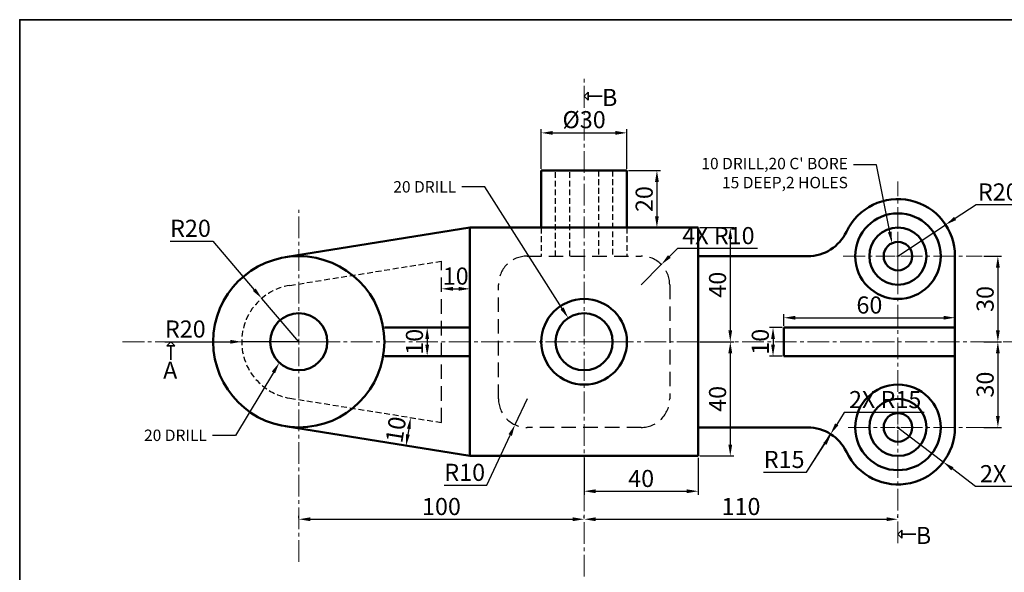
# Model space of a CAD drawing. Units: millimetres. Extents: x 33 to 569, y -180 to 232.
# Tile 2 of 3: x 33 to 378, y 39 to 232. Entities that reach past the tile are written whole.
import ezdxf
from ezdxf import colors
from ezdxf.entities.mleader import LeaderData, LeaderLine
from ezdxf.math import Vec2, Vec3

# ---------------------------------------------------------------- set-up
doc = ezdxf.new("R2010")
doc.units = ezdxf.units.MM
doc.header["$LTSCALE"] = 0.4
doc.linetypes.add('CENTER2', pattern=[28.575, 19.05, -3.175, 3.175, -3.175])
doc.linetypes.add('DASHED', pattern=[19.05, 12.7, -6.35])
for name, color, linetype, lineweight in [('M-CNTR', 1, 'CENTER2', 18), ('M-DIMS', 2, 'Continuous', 25), ('M-HIDN', 4, 'DASHED', 25), ('M-OUTL', 7, 'Continuous', 50), ('M-SECT', 6, 'Continuous', 35), ('M-TEXT', 3, 'Continuous', 25), ('M-TTLB', 7, 'Continuous', 35)]:
    doc.layers.add(name, color=color, linetype=linetype, lineweight=lineweight)
doc.styles.get("Standard").update_dxf_attribs({"font": 'arial.ttf'})
doc.dimstyles.new('ISO-25', dxfattribs={"dimtxt": 6, "dimasz": 4, "dimexe": 1.25, "dimexo": 0.625, "dimtad": 1, "dimtoh": 1, "dimdec": 0, "dimtxsty": 'Standard', "dimcen": 2.5, "dimadec": 0, "dimazin": 0, "dimtfac": 1, "dimtdec": 0, "dimtmove": 0, "dimatfit": 3, "dimfxl": 1, "dimarcsym": 0})

# ---------------------------------------------------------------- blocks, each defined once
blk = doc.blocks.new('*U1')
at = {"layer": 'M-CNTR', "color": 0, "transparency": 16777216}
blk.add_line((-161.75, 0), (175, 0), dxfattribs=at)
blk = doc.blocks.new('*U2')
at = {"layer": 'M-CNTR', "color": 0, "transparency": 16777216}
for p, q in [((0, 2), (0, 92.17)), ((-13.5, 0), (-2, 0)), ((2, 0), (13.5, 0)), ((0, -219.39), (0, -2))]:
    blk.add_line(p, q, dxfattribs=at)
at = {"layer": 'M-CNTR', "color": 0, "linetype": 'Continuous', "transparency": 16777216}
for p, q in [((-1, 0), (1, 0)), ((0, -1), (0, 1))]:
    blk.add_line(p, q, dxfattribs=at)
blk = doc.blocks.new('*U3')
at = {"layer": 'M-CNTR', "color": 0, "transparency": 16777216}
for p, q in [((0, 1), (0, 86.19)), ((-17.49, 0), (-1, 0)), ((1, 0), (30.13, 0)), ((0, -40.58), (0, -1))]:
    blk.add_line(p, q, dxfattribs=at)
at = {"layer": 'M-CNTR', "color": 0, "linetype": 'Continuous', "transparency": 16777216}
for p, q in [((-0.5, 0), (0.5, 0)), ((0, -0.5), (0, 0.5))]:
    blk.add_line(p, q, dxfattribs=at)
blk = doc.blocks.new('*D4')
at = {"layer": 'Defpoints', "color": 0, "ltscale": 0.4, "transparency": 16777216}
for p in [(245.35, 179.63), (245.35, 159.63), (255.87, 159.63)]:
    blk.add_point(p, dxfattribs=at)
at = {"layer": 'M-DIMS', "color": 0, "lineweight": -2, "ltscale": 0.4, "transparency": 16777216}
for p, q in [((245.97, 179.63), (257.12, 179.63)), ((255.87, 175.63), (255.87, 163.63)), ((245.97, 159.63), (257.12, 159.63))]:
    blk.add_line(p, q, dxfattribs=at)
at = {"layer": 'M-DIMS', "color": 0, "ltscale": 0.4, "transparency": 16777216}
for points in [[(255.2, 175.63), (256.54, 175.63), (255.87, 179.63)], [(255.2, 163.63), (256.54, 163.63), (255.87, 159.63)]]:
    blk.add_solid(points, dxfattribs=at)
at = {"layer": 'M-DIMS', "color": 0, "ltscale": 0.4, "transparency": 16777216, "insert": (252.18, 169.63), "char_height": 6, "attachment_point": 5, "rotation": 90}
blk.add_mtext('20', dxfattribs=at)
blk = doc.blocks.new('*D5')
at = {"layer": 'Defpoints', "color": 0, "ltscale": 0.4, "transparency": 16777216}
for p in [(245.35, 192.83), (215.35, 179.63), (245.35, 179.63)]:
    blk.add_point(p, dxfattribs=at)
at = {"layer": 'M-DIMS', "color": 0, "lineweight": -2, "ltscale": 0.4, "transparency": 16777216}
for p, q in [((215.35, 180.25), (215.35, 194.08)), ((245.35, 180.25), (245.35, 194.08)), ((219.35, 192.83), (241.35, 192.83))]:
    blk.add_line(p, q, dxfattribs=at)
at = {"layer": 'M-DIMS', "color": 0, "ltscale": 0.4, "transparency": 16777216}
for points in [[(219.35, 193.49), (219.35, 192.16), (215.35, 192.83)], [(241.35, 193.49), (241.35, 192.16), (245.35, 192.83)]]:
    blk.add_solid(points, dxfattribs=at)
at = {"layer": 'M-DIMS', "color": 0, "ltscale": 0.4, "transparency": 16777216, "insert": (230.35, 196.68), "char_height": 6, "attachment_point": 5}
blk.add_mtext('%%C30', dxfattribs=at)
blk = doc.blocks.new('*D6')
at = {"layer": 'Defpoints', "color": 0, "ltscale": 0.4, "transparency": 16777216}
for p in [(180.35, 138.19), (190.35, 138.19), (190.35, 138.19)]:
    blk.add_point(p, dxfattribs=at)
at = {"layer": 'M-DIMS', "color": 0, "lineweight": -2, "ltscale": 0.4, "transparency": 16777216}
for p, q in [((180.35, 138.82), (180.35, 139.44)), ((184.35, 138.19), (186.35, 138.19)), ((190.35, 138.82), (190.35, 139.44))]:
    blk.add_line(p, q, dxfattribs=at)
at = {"layer": 'M-DIMS', "color": 0, "ltscale": 0.4, "transparency": 16777216}
for points in [[(184.35, 138.86), (184.35, 137.52), (180.35, 138.19)], [(186.35, 138.86), (186.35, 137.52), (190.35, 138.19)]]:
    blk.add_solid(points, dxfattribs=at)
at = {"layer": 'M-DIMS', "color": 0, "ltscale": 0.4, "transparency": 16777216, "insert": (185.35, 141.88), "char_height": 6, "attachment_point": 5}
blk.add_mtext('10', dxfattribs=at)
blk = doc.blocks.new('*D7')
at = {"layer": 'Defpoints', "color": 0, "ltscale": 0.4, "transparency": 16777216}
for p in [(175.35, 124.63), (175.35, 114.63), (175.35, 114.63)]:
    blk.add_point(p, dxfattribs=at)
at = {"layer": 'M-DIMS', "color": 0, "lineweight": -2, "ltscale": 0.4, "transparency": 16777216}
for p, q in [((175.97, 124.63), (176.6, 124.63)), ((175.35, 120.63), (175.35, 118.63)), ((175.97, 114.63), (176.6, 114.63))]:
    blk.add_line(p, q, dxfattribs=at)
at = {"layer": 'M-DIMS', "color": 0, "ltscale": 0.4, "transparency": 16777216}
for points in [[(174.68, 120.63), (176.02, 120.63), (175.35, 124.63)], [(174.68, 118.63), (176.02, 118.63), (175.35, 114.63)]]:
    blk.add_solid(points, dxfattribs=at)
at = {"layer": 'M-DIMS', "color": 0, "ltscale": 0.4, "transparency": 16777216, "insert": (171.66, 119.63), "char_height": 6, "attachment_point": 5, "rotation": 90}
blk.add_mtext('10', dxfattribs=at)
blk = doc.blocks.new('*D8')
at = {"layer": 'Defpoints', "color": 0, "ltscale": 0.4, "transparency": 16777216}
for p in [(270.35, 159.63), (270.35, 119.63), (281.59, 119.63)]:
    blk.add_point(p, dxfattribs=at)
at = {"layer": 'M-DIMS', "color": 0, "lineweight": -2, "ltscale": 0.4, "transparency": 16777216}
for p, q in [((270.97, 159.63), (282.84, 159.63)), ((281.59, 155.63), (281.59, 123.63)), ((270.97, 119.63), (282.84, 119.63))]:
    blk.add_line(p, q, dxfattribs=at)
at = {"layer": 'M-DIMS', "color": 0, "ltscale": 0.4, "transparency": 16777216}
for points in [[(280.92, 155.63), (282.25, 155.63), (281.59, 159.63)], [(280.92, 123.63), (282.25, 123.63), (281.59, 119.63)]]:
    blk.add_solid(points, dxfattribs=at)
at = {"layer": 'M-DIMS', "color": 0, "ltscale": 0.4, "transparency": 16777216, "insert": (277.9, 139.63), "char_height": 6, "attachment_point": 5, "rotation": 90}
blk.add_mtext('40', dxfattribs=at)
blk = doc.blocks.new('*D9')
at = {"layer": 'Defpoints', "color": 0, "ltscale": 0.4, "transparency": 16777216}
for p in [(270.35, 119.63), (270.35, 79.63), (281.59, 79.63)]:
    blk.add_point(p, dxfattribs=at)
at = {"layer": 'M-DIMS', "color": 0, "lineweight": -2, "ltscale": 0.4, "transparency": 16777216}
for p, q in [((270.97, 119.63), (282.84, 119.63)), ((281.59, 115.63), (281.59, 83.63)), ((270.97, 79.63), (282.84, 79.63))]:
    blk.add_line(p, q, dxfattribs=at)
at = {"layer": 'M-DIMS', "color": 0, "ltscale": 0.4, "transparency": 16777216}
for points in [[(280.92, 115.63), (282.25, 115.63), (281.59, 119.63)], [(280.92, 83.63), (282.25, 83.63), (281.59, 79.63)]]:
    blk.add_solid(points, dxfattribs=at)
at = {"layer": 'M-DIMS', "color": 0, "ltscale": 0.4, "transparency": 16777216, "insert": (277.9, 99.63), "char_height": 6, "attachment_point": 5, "rotation": 90}
blk.add_mtext('40', dxfattribs=at)
blk = doc.blocks.new('*D10')
at = {"layer": 'Defpoints', "color": 0, "ltscale": 0.4, "transparency": 16777216}
for p in [(300.35, 124.63), (296.57, 114.63), (300.35, 114.63)]:
    blk.add_point(p, dxfattribs=at)
at = {"layer": 'M-DIMS', "color": 0, "lineweight": -2, "ltscale": 0.4, "transparency": 16777216}
for p, q in [((299.72, 124.63), (295.32, 124.63)), ((296.57, 120.63), (296.57, 118.63)), ((299.72, 114.63), (295.32, 114.63))]:
    blk.add_line(p, q, dxfattribs=at)
at = {"layer": 'M-DIMS', "color": 0, "ltscale": 0.4, "transparency": 16777216}
for points in [[(295.9, 120.63), (297.24, 120.63), (296.57, 124.63)], [(295.9, 118.63), (297.24, 118.63), (296.57, 114.63)]]:
    blk.add_solid(points, dxfattribs=at)
at = {"layer": 'M-DIMS', "color": 0, "ltscale": 0.4, "transparency": 16777216, "insert": (292.88, 119.63), "char_height": 6, "attachment_point": 5, "rotation": 90}
blk.add_mtext('10', dxfattribs=at)
blk = doc.blocks.new('*D11')
at = {"layer": 'Defpoints', "color": 0, "ltscale": 0.4, "transparency": 16777216}
for p in [(360.35, 128.05), (300.35, 124.63), (360.35, 124.63)]:
    blk.add_point(p, dxfattribs=at)
at = {"layer": 'M-DIMS', "color": 0, "lineweight": -2, "ltscale": 0.4, "transparency": 16777216}
for p, q in [((300.35, 125.25), (300.35, 129.3)), ((304.35, 128.05), (356.35, 128.05)), ((360.35, 125.25), (360.35, 129.3))]:
    blk.add_line(p, q, dxfattribs=at)
at = {"layer": 'M-DIMS', "color": 0, "ltscale": 0.4, "transparency": 16777216}
for points in [[(304.35, 128.72), (304.35, 127.39), (300.35, 128.05)], [(356.35, 128.72), (356.35, 127.39), (360.35, 128.05)]]:
    blk.add_solid(points, dxfattribs=at)
at = {"layer": 'M-DIMS', "color": 0, "ltscale": 0.4, "transparency": 16777216, "insert": (330.35, 131.74), "char_height": 6, "attachment_point": 5}
blk.add_mtext('60', dxfattribs=at)
blk = doc.blocks.new('*D12')
at = {"layer": 'Defpoints', "color": 0, "ltscale": 0.4, "transparency": 16777216}
for p in [(230.35, 79.63), (270.35, 79.63), (270.35, 67.27)]:
    blk.add_point(p, dxfattribs=at)
at = {"layer": 'M-DIMS', "color": 0, "lineweight": -2, "ltscale": 0.4, "transparency": 16777216}
for p, q in [((230.35, 79), (230.35, 66.02)), ((270.35, 79), (270.35, 66.02)), ((234.35, 67.27), (266.35, 67.27))]:
    blk.add_line(p, q, dxfattribs=at)
at = {"layer": 'M-DIMS', "color": 0, "ltscale": 0.4, "transparency": 16777216}
for points in [[(234.35, 67.93), (234.35, 66.6), (230.35, 67.27)], [(266.35, 67.93), (266.35, 66.6), (270.35, 67.27)]]:
    blk.add_solid(points, dxfattribs=at)
at = {"layer": 'M-DIMS', "color": 0, "ltscale": 0.4, "transparency": 16777216, "insert": (250.35, 70.95), "char_height": 6, "attachment_point": 5}
blk.add_mtext('40', dxfattribs=at)
blk = doc.blocks.new('*U13')
at = {"layer": 'M-CNTR', "color": 0, "transparency": 16777216}
for p, q in [((0, 2), (0, 46.22)), ((-13.5, 0), (-2, 0)), ((2, 0), (13.5, 0)), ((0, -77.08), (0, -2))]:
    blk.add_line(p, q, dxfattribs=at)
at = {"layer": 'M-CNTR', "color": 0, "linetype": 'Continuous', "transparency": 16777216}
for p, q in [((-1, 0), (1, 0)), ((0, -1), (0, 1))]:
    blk.add_line(p, q, dxfattribs=at)
blk = doc.blocks.new('*D14')
at = {"layer": 'Defpoints', "color": 0, "ltscale": 0.4, "transparency": 16777216}
for p in [(130.35, 57.22), (230.35, 57.45), (230.35, 57.22)]:
    blk.add_point(p, dxfattribs=at)
at = {"layer": 'M-DIMS', "color": 0, "lineweight": -2, "ltscale": 0.4, "transparency": 16777216}
for p, q in [((130.35, 57.85), (130.35, 58.7)), ((230.35, 57.85), (230.35, 58.7)), ((134.35, 57.45), (226.35, 57.45))]:
    blk.add_line(p, q, dxfattribs=at)
at = {"layer": 'M-DIMS', "color": 0, "ltscale": 0.4, "transparency": 16777216}
for points in [[(134.35, 58.12), (134.35, 56.78), (130.35, 57.45)], [(226.35, 58.12), (226.35, 56.78), (230.35, 57.45)]]:
    blk.add_solid(points, dxfattribs=at)
at = {"layer": 'M-DIMS', "color": 0, "ltscale": 0.4, "transparency": 16777216, "insert": (180.35, 61.14), "char_height": 6, "attachment_point": 5}
blk.add_mtext('100', dxfattribs=at)
blk = doc.blocks.new('*D15')
at = {"layer": 'Defpoints', "color": 0, "ltscale": 0.4, "transparency": 16777216}
for p in [(230.35, 57.45), (340.35, 57.45), (340.35, 57.45)]:
    blk.add_point(p, dxfattribs=at)
at = {"layer": 'M-DIMS', "color": 0, "lineweight": -2, "ltscale": 0.4, "transparency": 16777216}
for p, q in [((230.35, 58.08), (230.35, 58.7)), ((340.35, 58.08), (340.35, 58.7)), ((234.35, 57.45), (336.35, 57.45))]:
    blk.add_line(p, q, dxfattribs=at)
at = {"layer": 'M-DIMS', "color": 0, "ltscale": 0.4, "transparency": 16777216}
for points in [[(234.35, 58.12), (234.35, 56.78), (230.35, 57.45)], [(336.35, 58.12), (336.35, 56.78), (340.35, 57.45)]]:
    blk.add_solid(points, dxfattribs=at)
at = {"layer": 'M-DIMS', "color": 0, "ltscale": 0.4, "transparency": 16777216, "insert": (285.35, 61.14), "char_height": 6, "attachment_point": 5}
blk.add_mtext('110', dxfattribs=at)
blk = doc.blocks.new('*U16')
at = {"layer": 'M-CNTR', "color": 0, "transparency": 16777216}
for p, q in [((0, 1), (0, 8.5)), ((-19.15, 0), (-1, 0)), ((1, 0), (29.5, 0)), ((0, -8.5), (0, -1))]:
    blk.add_line(p, q, dxfattribs=at)
at = {"layer": 'M-CNTR', "color": 0, "linetype": 'Continuous', "transparency": 16777216}
for p, q in [((-0.5, 0), (0.5, 0)), ((0, -0.5), (0, 0.5))]:
    blk.add_line(p, q, dxfattribs=at)
blk = doc.blocks.new('*D17')
at = {"layer": 'Defpoints', "color": 0, "ltscale": 0.4, "transparency": 16777216}
for p in [(369.85, 149.63), (369.85, 119.63), (375.38, 119.63)]:
    blk.add_point(p, dxfattribs=at)
at = {"layer": 'M-DIMS', "color": 0, "lineweight": -2, "ltscale": 0.4, "transparency": 16777216}
for p, q in [((370.47, 149.63), (376.63, 149.63)), ((375.38, 145.63), (375.38, 123.63)), ((370.47, 119.63), (376.63, 119.63))]:
    blk.add_line(p, q, dxfattribs=at)
at = {"layer": 'M-DIMS', "color": 0, "ltscale": 0.4, "transparency": 16777216}
for points in [[(374.71, 145.63), (376.04, 145.63), (375.38, 149.63)], [(374.71, 123.63), (376.04, 123.63), (375.38, 119.63)]]:
    blk.add_solid(points, dxfattribs=at)
at = {"layer": 'M-DIMS', "color": 0, "ltscale": 0.4, "transparency": 16777216, "insert": (371.69, 134.63), "char_height": 6, "attachment_point": 5, "rotation": 90}
blk.add_mtext('30', dxfattribs=at)
blk = doc.blocks.new('*D18')
at = {"layer": 'Defpoints', "color": 0, "ltscale": 0.4, "transparency": 16777216}
for p in [(369.85, 119.63), (369.85, 89.63), (375.38, 89.63)]:
    blk.add_point(p, dxfattribs=at)
at = {"layer": 'M-DIMS', "color": 0, "lineweight": -2, "ltscale": 0.4, "transparency": 16777216}
for p, q in [((370.47, 119.63), (376.63, 119.63)), ((375.38, 115.63), (375.38, 93.63)), ((370.47, 89.63), (376.63, 89.63))]:
    blk.add_line(p, q, dxfattribs=at)
at = {"layer": 'M-DIMS', "color": 0, "ltscale": 0.4, "transparency": 16777216}
for points in [[(374.71, 115.63), (376.04, 115.63), (375.38, 119.63)], [(374.71, 93.63), (376.04, 93.63), (375.38, 89.63)]]:
    blk.add_solid(points, dxfattribs=at)
at = {"layer": 'M-DIMS', "color": 0, "ltscale": 0.4, "transparency": 16777216, "insert": (371.69, 104.63), "char_height": 6, "attachment_point": 5, "rotation": 90}
blk.add_mtext('30', dxfattribs=at)
blk = doc.blocks.new('*D19')
at = {"layer": 'Defpoints', "color": 0, "ltscale": 0.4, "transparency": 16777216}
for p in [(357.05, 160.63), (340.35, 149.63)]:
    blk.add_point(p, dxfattribs=at)
at = {"layer": 'M-DIMS', "color": 0, "lineweight": -2, "ltscale": 0.4, "transparency": 16777216}
for p, q in [((367.74, 167.66), (360.4, 162.83)), ((382.68, 167.66), (367.74, 167.66)), ((340.35, 149.63), (357.05, 160.63))]:
    blk.add_line(p, q, dxfattribs=at)
at = {"layer": 'M-DIMS', "color": 0, "ltscale": 0.4, "transparency": 16777216}
blk.add_solid([(360.03, 163.38), (360.76, 162.27), (357.05, 160.63)], dxfattribs=at)
at = {"layer": 'M-DIMS', "color": 0, "ltscale": 0.4, "transparency": 16777216, "insert": (375.52, 171.35), "char_height": 6, "attachment_point": 5}
blk.add_mtext('R20', dxfattribs=at)
blk = doc.blocks.new('*D20')
at = {"layer": 'Defpoints', "color": 0, "ltscale": 0.4, "transparency": 16777216}
for p in [(210.35, 99.63), (206.13, 90.56)]:
    blk.add_point(p, dxfattribs=at)
at = {"layer": 'M-DIMS', "color": 0, "lineweight": -2, "ltscale": 0.4, "transparency": 16777216}
for p, q in [((210.35, 99.63), (206.13, 90.56)), ((196.28, 69.42), (204.44, 86.94)), ((181.34, 69.42), (196.28, 69.42))]:
    blk.add_line(p, q, dxfattribs=at)
at = {"layer": 'M-DIMS', "color": 0, "ltscale": 0.4, "transparency": 16777216}
blk.add_solid([(203.84, 87.22), (205.04, 86.66), (206.13, 90.56)], dxfattribs=at)
at = {"layer": 'M-DIMS', "color": 0, "ltscale": 0.4, "transparency": 16777216, "insert": (188.5, 73.11), "char_height": 6, "attachment_point": 5}
blk.add_mtext('R10', dxfattribs=at)
blk = doc.blocks.new('*D21')
at = {"layer": 'Defpoints', "color": 0, "ltscale": 0.4, "transparency": 16777216}
for p in [(316.92, 87.19), (308.73, 74.63)]:
    blk.add_point(p, dxfattribs=at)
at = {"layer": 'M-DIMS', "color": 0, "lineweight": -2, "ltscale": 0.4, "transparency": 16777216}
for p, q in [((308.28, 73.95), (314.74, 83.84)), ((293.27, 73.95), (308.28, 73.95))]:
    blk.add_line(p, q, dxfattribs=at)
at = {"layer": 'M-DIMS', "color": 0, "ltscale": 0.4, "transparency": 16777216}
blk.add_solid([(314.18, 84.21), (315.29, 83.48), (316.92, 87.19)], dxfattribs=at)
at = {"layer": 'M-DIMS', "color": 0, "ltscale": 0.4, "transparency": 16777216, "insert": (300.47, 77.63), "char_height": 6, "attachment_point": 5}
blk.add_mtext('R15', dxfattribs=at)
blk = doc.blocks.new('*D22')
at = {"layer": 'Defpoints', "color": 0, "ltscale": 0.4, "transparency": 16777216}
for p in [(117.36, 134.83), (130.35, 119.63)]:
    blk.add_point(p, dxfattribs=at)
at = {"layer": 'M-DIMS', "color": 0, "lineweight": -2, "ltscale": 0.4, "transparency": 16777216}
for p, q in [((85.24, 154.93), (100.18, 154.93)), ((100.18, 154.93), (114.76, 137.87)), ((130.35, 119.63), (117.36, 134.83))]:
    blk.add_line(p, q, dxfattribs=at)
at = {"layer": 'M-DIMS', "color": 0, "ltscale": 0.4, "transparency": 16777216}
blk.add_solid([(115.26, 138.31), (114.25, 137.44), (117.36, 134.83)], dxfattribs=at)
at = {"layer": 'M-DIMS', "color": 0, "ltscale": 0.4, "transparency": 16777216, "insert": (92.39, 158.62), "char_height": 6, "attachment_point": 5}
blk.add_mtext('R20', dxfattribs=at)
blk = doc.blocks.new('*D23')
at = {"layer": 'Defpoints', "color": 0, "ltscale": 0.4, "transparency": 16777216}
for p in [(169.55, 93.09), (167.97, 83.22), (167.97, 83.22)]:
    blk.add_point(p, dxfattribs=at)
at = {"layer": 'M-DIMS', "color": 0, "lineweight": -2, "ltscale": 0.4, "transparency": 16777216}
for p, q in [((170.17, 92.99), (170.79, 92.89)), ((168.92, 89.14), (168.6, 87.17)), ((168.59, 83.12), (169.2, 83.02))]:
    blk.add_line(p, q, dxfattribs=at)
at = {"layer": 'M-DIMS', "color": 0, "ltscale": 0.4, "transparency": 16777216}
for points in [[(168.26, 89.25), (169.58, 89.04), (169.55, 93.09)], [(167.94, 87.27), (169.26, 87.06), (167.97, 83.22)]]:
    blk.add_solid(points, dxfattribs=at)
at = {"layer": 'M-DIMS', "color": 0, "ltscale": 0.4, "transparency": 16777216, "insert": (165.12, 88.74), "char_height": 6, "attachment_point": 5, "rotation": 80.8938}
blk.add_mtext('10', dxfattribs=at)
blk = doc.blocks.new('SECTION-ARROW')
at = {"ltscale": 0.4}
for p, q in [((0, 1.41), (1.41, 2.83)), ((0, 1.41), (1.41, 0)), ((1.41, 2.83), (1.41, 0)), ((1.41, 1.41), (6.28, 1.41))]:
    blk.add_line(p, q, dxfattribs=at)
blk = doc.blocks.new('CBORE-M10')
for radius in [15, 10, 5]:
    blk.add_circle((15, 15), radius)
blk = doc.blocks.new('*D49')
at = {"layer": 'Defpoints', "color": 0, "ltscale": 0.4, "transparency": 16777216}
for p in [(340.35, 89.63), (356.26, 77.51)]:
    blk.add_point(p, dxfattribs=at)
at = {"layer": 'M-DIMS', "color": 0, "lineweight": -2, "ltscale": 0.4, "transparency": 16777216}
for p, q in [((340.35, 89.63), (356.26, 77.51)), ((367.5, 68.95), (359.44, 75.09)), ((395.43, 68.95), (367.5, 68.95))]:
    blk.add_line(p, q, dxfattribs=at)
at = {"layer": 'M-DIMS', "color": 0, "ltscale": 0.4, "transparency": 16777216}
blk.add_solid([(359.85, 75.62), (359.04, 74.56), (356.26, 77.51)], dxfattribs=at)
at = {"layer": 'M-DIMS', "color": 0, "ltscale": 0.4, "transparency": 16777216, "insert": (381.78, 72.64), "char_height": 6, "attachment_point": 5}
blk.add_mtext('2X R20', dxfattribs=at)
blk = doc.blocks.new('*D50')
at = {"layer": 'Defpoints', "color": 0, "ltscale": 0.4, "transparency": 16777216}
for p in [(316.74, 87.31), (308.73, 74.63)]:
    blk.add_point(p, dxfattribs=at)
at = {"layer": 'M-DIMS', "color": 0, "lineweight": -2, "ltscale": 0.4, "transparency": 16777216}
for p, q in [((321.56, 94.91), (318.88, 90.69)), ((349.56, 94.91), (321.56, 94.91)), ((308.73, 74.63), (316.74, 87.31))]:
    blk.add_line(p, q, dxfattribs=at)
at = {"layer": 'M-DIMS', "color": 0, "ltscale": 0.4, "transparency": 16777216}
blk.add_solid([(318.32, 91.04), (319.45, 90.33), (316.74, 87.31)], dxfattribs=at)
at = {"layer": 'M-DIMS', "color": 0, "ltscale": 0.4, "transparency": 16777216, "insert": (335.87, 98.6), "char_height": 6, "attachment_point": 5}
blk.add_mtext('2X R15', dxfattribs=at)
blk = doc.blocks.new('*D51')
at = {"layer": 'Defpoints', "color": 0, "ltscale": 0.4, "transparency": 16777216}
for p in [(257.42, 146.7), (250.35, 139.63)]:
    blk.add_point(p, dxfattribs=at)
at = {"layer": 'M-DIMS', "color": 0, "lineweight": -2, "ltscale": 0.4, "transparency": 16777216}
for p, q in [((263.08, 152.36), (260.25, 149.53)), ((291.15, 152.36), (263.08, 152.36)), ((250.35, 139.63), (257.42, 146.7))]:
    blk.add_line(p, q, dxfattribs=at)
at = {"layer": 'M-DIMS', "color": 0, "ltscale": 0.4, "transparency": 16777216}
blk.add_solid([(259.78, 150), (260.72, 149.06), (257.42, 146.7)], dxfattribs=at)
at = {"layer": 'M-DIMS', "color": 0, "ltscale": 0.4, "transparency": 16777216, "insert": (277.43, 156.05), "char_height": 6, "attachment_point": 5}
blk.add_mtext('4X R10', dxfattribs=at)
blk = doc.blocks.new('*D52')
at = {"layer": 'Defpoints', "color": 0, "ltscale": 0.4, "transparency": 16777216}
for p in [(110.35, 119.63), (130.35, 119.63)]:
    blk.add_point(p, dxfattribs=at)
at = {"layer": 'M-DIMS', "color": 0, "lineweight": -2, "ltscale": 0.4, "transparency": 16777216}
for p, q in [((83.41, 119.63), (98.35, 119.63)), ((98.35, 119.63), (106.35, 119.63)), ((130.35, 119.63), (110.35, 119.63))]:
    blk.add_line(p, q, dxfattribs=at)
at = {"layer": 'M-DIMS', "color": 0, "ltscale": 0.4, "transparency": 16777216}
blk.add_solid([(106.35, 120.3), (106.35, 118.96), (110.35, 119.63)], dxfattribs=at)
at = {"layer": 'M-DIMS', "color": 0, "ltscale": 0.4, "transparency": 16777216, "insert": (90.57, 123.32), "char_height": 6, "attachment_point": 5}
blk.add_mtext('R20', dxfattribs=at)

msp = doc.modelspace()

# ---------------------------------------------------------------- linework, layer by layer
at = {"layer": 'M-HIDN', "ltscale": 0.4}
for p, q in [((220.35, 149.63), (220.35, 179.63)), ((225.35, 149.63), (225.35, 179.63)), ((235.35, 179.63), (235.35, 149.63)), ((240.35, 179.63), (240.35, 149.63)), ((215.35, 159.63), (215.35, 149.63)), ((245.35, 159.63), (245.35, 149.63)), ((127.18, 139.38), (180.35, 147.9)), ((127.18, 99.88), (180.35, 91.36))]:
    msp.add_line(p, q, dxfattribs=at)
at = {"layer": 'M-HIDN'}
msp.add_line((180.35, 91.36), (180.35, 147.9), dxfattribs=at)
msp.add_lwpolyline([(210.35, 149.63), (250.35, 149.63, -0.414214), (260.35, 139.63), (260.35, 99.63, -0.414214), (250.35, 89.63), (210.35, 89.63, -0.414214), (200.35, 99.63), (200.35, 139.63, -0.414214)], format="xyb", close=True, dxfattribs=at)
at = {"layer": 'M-HIDN', "ltscale": 0.4}
msp.add_arc((130.35, 119.63), 20, 99.1062, 260.8938, dxfattribs=at)
at = {"layer": 'M-OUTL', "ltscale": 0.4}
for p, q in [((215.35, 179.63), (245.35, 179.63)), ((215.35, 159.63), (215.35, 179.63)), ((245.35, 179.63), (245.35, 159.63)), ((125.6, 149.25), (190.35, 159.63)), ((245.35, 159.63), (215.35, 159.63)), ((160.35, 124.63), (190.35, 124.63)), ((300.35, 114.63), (300.35, 124.63)), ((160.35, 114.63), (190.35, 114.63)), ((125.6, 90.01), (190.35, 79.63))]:
    msp.add_line(p, q, dxfattribs=at)
at = {"layer": 'M-OUTL'}
for p, q in [((190.35, 159.63), (270.35, 159.63)), ((190.35, 79.63), (190.35, 159.63)), ((270.35, 159.63), (270.35, 79.63)), ((308.73, 149.63), (270.35, 149.63)), ((360.35, 149.63), (360.35, 89.63)), ((300.35, 124.63), (300.35, 114.63)), ((360.35, 124.63), (300.35, 124.63)), ((360.35, 114.63), (360.35, 124.63)), ((300.35, 114.63), (360.35, 114.63)), ((308.73, 89.63), (270.35, 89.63)), ((270.35, 79.63), (190.35, 79.63))]:
    msp.add_line(p, q, dxfattribs=at)
for centre, radius in [((130.35, 119.63), 30), ((230.35, 119.63), 15), ((230.35, 119.63), 10)]:
    msp.add_circle(centre, radius, dxfattribs=at)
at = {"layer": 'M-OUTL', "ltscale": 0.4}
msp.add_circle((130.35, 119.63), 10, dxfattribs=at)
at = {"layer": 'M-OUTL'}
for centre, radius, start, end in [((340.35, 149.63), 20, 0, 154.6231), ((308.73, 164.63), 15, 270, 334.6231), ((308.73, 74.63), 15, 25.3769, 90), ((340.35, 89.63), 20, 205.3769, 0)]:
    msp.add_arc(centre, radius, start, end, dxfattribs=at)
at = {"layer": 'M-TTLB', "ltscale": 0.4}
msp.add_lwpolyline([(568.64, -179.82), (32.52, -179.82), (32.52, 232.48), (568.64, 232.48)], close=True, dxfattribs=at)

# ---------------------------------------------------------------- block references
at = {"layer": 'M-CNTR'}
for name, p in [('*U2', (230.35, 119.63)), ('*U3', (340.35, 89.63)), ('*U13', (130.35, 119.63)), ('*U16', (340.35, 149.63)), ('*U1', (230.35, 119.63))]:
    msp.add_blockref(name, p, dxfattribs=at)
at = {"layer": 'M-OUTL'}
for p in [(325.35, 134.63), (325.35, 74.63)]:
    msp.add_blockref('CBORE-M10', p, dxfattribs=at)
at = {"layer": 'M-SECT'}
for p in [(230.35, 204.26), (340.35, 50.8)]:
    msp.add_blockref('SECTION-ARROW', p, dxfattribs=at)
at = {"layer": 'M-SECT', "rotation": 270.0000000000007}
msp.add_blockref('SECTION-ARROW', (84.09, 119.63), dxfattribs=at)

# ---------------------------------------------------------------- texts
at = {"layer": 'M-TEXT', "ltscale": 0.4, "char_height": 6, "attachment_point": 1}
for s, insert in [('B', (236.63, 208.23)), ('A', (82.8, 112.65)), ('B', (346.63, 54.77))]:
    msp.add_mtext_dynamic_manual_height_columns(s, width=4.1924, gutter_width=12.5, heights=[0], dxfattribs=dict(at, insert=insert))

# ---------------------------------------------------------------- dimensions: what is measured, and where the dimension line sits
at = {"layer": 'M-DIMS', "ltscale": 0.4}
dim = msp.add_linear_dim(base=(245.35, 192.83), p1=(215.35, 179.63), p2=(245.35, 179.63), text='%%C<>', dimstyle='ISO-25', override={"dimclrd": 0, "dimclre": 0, "dimclrt": 0}, dxfattribs=at)
dim.commit()
dim.dimension.update_dxf_attribs({"geometry": '*D5', "text_midpoint": (230.35, 192.83), "dimtype": 160})
for base, p1, p2, picture, middle in [((255.87, 159.63), (245.35, 179.63), (245.35, 159.63), '*D4', (252.18, 169.63)), ((281.59, 119.63), (270.35, 159.63), (270.35, 119.63), '*D8', (277.9, 139.63)), ((375.38, 119.63), (369.85, 149.63), (369.85, 119.63), '*D17', (371.69, 134.63)), ((175.35, 114.63), (175.35, 124.63), (175.35, 114.63), '*D7', (171.66, 119.63)), ((296.57, 114.63), (300.35, 124.63), (300.35, 114.63), '*D10', (292.88, 119.63)), ((281.59, 79.63), (270.35, 119.63), (270.35, 79.63), '*D9', (277.9, 99.63)), ((375.38, 89.63), (369.85, 119.63), (369.85, 89.63), '*D18', (371.69, 104.63))]:
    dim = msp.add_linear_dim(base=base, p1=p1, p2=p2, angle=90, dimstyle='ISO-25', override={"dimclrd": 0, "dimclre": 0, "dimclrt": 0}, dxfattribs=at)
    dim.commit()
    dim.dimension.update_dxf_attribs({"geometry": picture, "text_midpoint": middle})
for center, mpoint, override, picture, middle in [((340.35, 149.63), (357.05, 160.63), {"dimclrd": 0, "dimclre": 0, "dimclrt": 0}, '*D19', (375.52, 167.66)), ((130.35, 119.63), (117.36, 134.83), {"dimclrd": 0, "dimclre": 0, "dimclrt": 0}, '*D22', (92.39, 154.93)), ((130.35, 119.63), (110.35, 119.63), {"dimdec": 0, "dimlfac": 1, "dimrnd": 0, "dimzin": 0, "dimdsep": 46, "dimlunit": 2}, '*D52', (98.35, 119.63)), ((210.35, 99.63), (206.13, 90.56), {"dimclrd": 0, "dimclre": 0, "dimclrt": 0}, '*D20', (188.5, 69.42)), ((308.73, 74.63), (316.92, 87.19), {"dimclrd": 0, "dimclre": 0, "dimclrt": 0}, '*D21', (300.47, 73.95))]:
    dim = msp.add_radius_dim(center=center, mpoint=mpoint, dimstyle='ISO-25', override=override, dxfattribs=at)
    dim.commit()
    dim.dimension.update_dxf_attribs({"geometry": picture, "text_midpoint": middle, "dimtype": 164})
for center, mpoint, text, picture, middle in [((250.35, 139.63), (257.42, 146.7), '4X <>', '*D51', (277.43, 156.05)), ((340.35, 89.63), (356.26, 77.51), '2X <>', '*D49', (381.78, 72.64))]:
    dim = msp.add_radius_dim(center=center, mpoint=mpoint, text=text, dimstyle='ISO-25', override={"dimdec": 0, "dimlfac": 1, "dimrnd": 0, "dimzin": 0, "dimdsep": 46, "dimlunit": 2}, dxfattribs=at)
    dim.commit()
    dim.dimension.update_dxf_attribs({"geometry": picture, "text_midpoint": middle})
for base, p1, p2, picture, middle in [((190.35, 138.19), (180.35, 138.19), (190.35, 138.19), '*D6', (185.35, 141.88)), ((360.35, 128.05), (300.35, 124.63), (360.35, 124.63), '*D11', (330.35, 131.74)), ((270.35, 67.27), (230.35, 79.63), (270.35, 79.63), '*D12', (250.35, 70.95)), ((230.35, 57.45), (130.35, 57.22), (230.35, 57.22), '*D14', (180.35, 61.14)), ((340.35, 57.45), (230.35, 57.45), (340.35, 57.45), '*D15', (285.35, 61.14))]:
    dim = msp.add_linear_dim(base=base, p1=p1, p2=p2, dimstyle='ISO-25', override={"dimclrd": 0, "dimclre": 0, "dimclrt": 0}, dxfattribs=at)
    dim.commit()
    dim.dimension.update_dxf_attribs({"geometry": picture, "text_midpoint": middle})
dim = msp.add_radius_dim(center=(308.73, 74.63), mpoint=(316.74, 87.31), text='2X <>', dimstyle='ISO-25', override={"dimdec": 0, "dimlfac": 1, "dimrnd": 0, "dimzin": 0, "dimdsep": 46, "dimlunit": 2}, dxfattribs=at)
dim.commit()
dim.dimension.update_dxf_attribs({"geometry": '*D50', "text_midpoint": (335.87, 94.91), "dimtype": 164})
dim = msp.add_aligned_dim(p1=(169.55, 93.09), p2=(167.97, 83.22), distance=0, dimstyle='ISO-25', override={"dimclrd": 0, "dimclre": 0, "dimclrt": 0}, dxfattribs=at)
dim.commit()
dim.dimension.update_dxf_attribs({"geometry": '*D23', "text_midpoint": (165.12, 88.74)})

# ---------------------------------------------------------------- leaders
at = {"layer": 'M-TEXT', "ltscale": 0.4}
ml = msp.add_multileader_mtext('Standard', dxfattribs=at)
ml.set_content("10 DRILL,20 C' BORE\\P15 DEEP,2 HOLES", color=256)
ml.set_leader_properties()
ml.build(insert=Vec2(0, 0))
ctx = ml.context
ctx.base_point, ctx.plane_origin = Vec3(266.3, 181.68), Vec3(338.27, 154.18)
ctx.text_align_type = 2
notes = []
notes.append((ctx, [(0, (1, 1, 0), (332.81, 181.68), (-1, 0), 8, [(0, [(338.27, 154.18)], 0, [])])]))
ctx.mtext.insert, ctx.mtext.alignment, ctx.mtext.flow_direction = Vec3(322.81, 184.08), 3, 5
ml = msp.add_multileader_mtext('Standard', dxfattribs=at)
ml.set_content('20 DRILL', color=256)
ml.set_leader_properties()
ml.build(insert=Vec2(0, 0))
ctx = ml.context
ctx.base_point, ctx.plane_origin = Vec3(160.26, 173.89), Vec3(224.79, 127.94)
ctx.text_align_type = 2
notes.append((ctx, [(0, (1, 1, 0), (195.5, 173.89), (-1, 0), 8, [(0, [(224.79, 127.94)], 0, [])])]))
ctx.mtext.insert, ctx.mtext.alignment, ctx.mtext.flow_direction = Vec3(185.5, 175.93), 3, 5
ml = msp.add_multileader_mtext('Standard', dxfattribs=at)
ml.set_content('20 DRILL', color=256)
ml.set_leader_properties()
ml.build(insert=Vec2(0, 0))
ctx = ml.context
ctx.base_point, ctx.plane_origin = Vec3(72.88, 86.82), Vec3(123.53, 112.32)
ctx.text_align_type = 2
notes.append((ctx, [(0, (1, 1, 0), (108.13, 86.82), (-1, 0), 8, [(0, [(123.53, 112.32)], 0, [])])]))
ctx.mtext.insert, ctx.mtext.alignment, ctx.mtext.flow_direction = Vec3(98.13, 88.86), 3, 5
for ctx, leaders in notes:
    for number, flags, end, landing, length, lines in leaders:
        leader = LeaderData()
        leader.index, (leader.has_last_leader_line, leader.has_dogleg_vector, leader.attachment_direction) = number, flags
        leader.last_leader_point, leader.dogleg_vector, leader.dogleg_length = Vec3(end), Vec3(landing), length
        for number, points, colour, breaks in lines:
            line = LeaderLine()
            line.index, line.vertices, line.color, line.breaks = number, Vec3.list(points), colors.encode_raw_color(colour), breaks
            leader.lines.append(line)
        ctx.leaders.append(leader)

doc.saveas('drawing.dxf')
